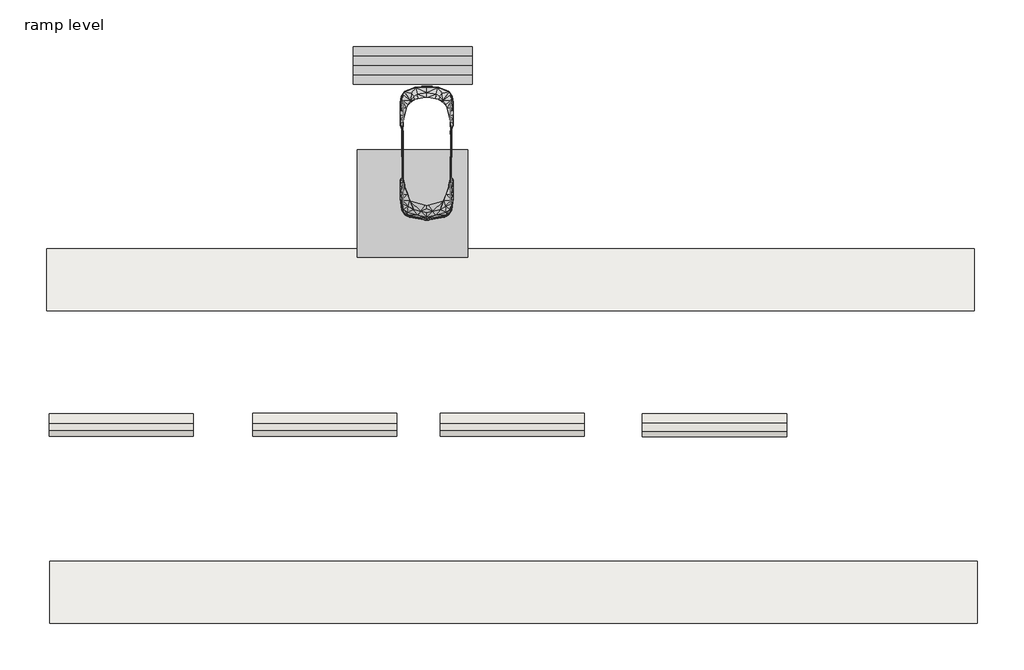
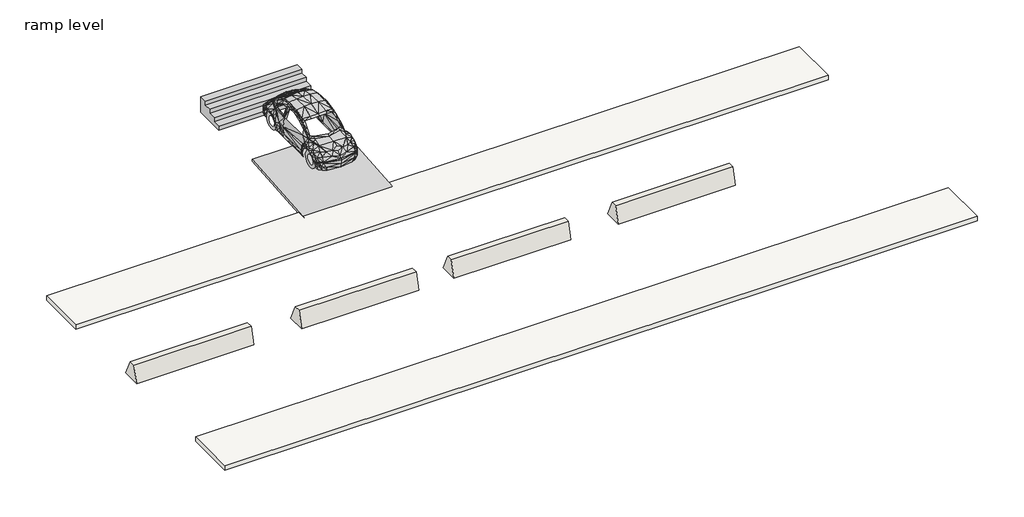
# One storey: 4 walls, 2 slabs, 1 furniture element, 1 proxy, 1 ramp.
"""IFC4 building model written with IfcOpenShell, lengths in millimetres."""

from ifc_helpers import new_model, si_unit, frame, origin, place, context, project, spatial, polyline, outline, extrude, transform, mapped, element, save
from components import rpc_beetle_rpc_beetle_31f8b51e, casework_2_casework_2_ff1f8355, ramp_2_4435543f, floors_1_floors_1_86c0a0b5, floors_2_floors_1_5c930e2b

model = new_model("IFC4")

# Units and contexts
model_context = context("Model", 3, world=origin())
ifc_project = project(units=[si_unit("LENGTHUNIT", "METRE", prefix="MILLI")], contexts=[model_context])

# Site, building, storey
site = spatial("IfcSite", under=ifc_project)
building = spatial("IfcBuilding", under=site)
storey = spatial("IfcBuildingStorey", under=building, Name="ramp level", Elevation=-304.8)

# Proxy
placement = place(None, origin())
rpc_beetle_rpc_beetle_shape = rpc_beetle_rpc_beetle_31f8b51e(model_context)
element("IfcBuildingElementProxy", 1, Name="RPC Beetle : RPC Beetle", ObjectType="RPC Beetle : RPC Beetle", at=placement, inside=storey, context=model_context, shape_type="MappedRepresentation", body=[
    mapped(rpc_beetle_rpc_beetle_shape, transform((25158.1789072, 4428.0409313, 0.0), x_axis=(-1.0, 0.0, 0.0), y_axis=(0.0, -1.0, 0.0), z_axis=(0.0, 0.0, 1.0))),
])

# Furniture
casework_2_casework_2_shape = casework_2_casework_2_ff1f8355(model_context)
element("IfcFurniture", 2, ObjectType="Casework 2 : Casework 2", at=placement, inside=storey, context=model_context, shape_type="MappedRepresentation", body=[
    mapped(casework_2_casework_2_shape, transform((0.0, -262.7690365, -6.2943409), x_axis=(1.0, 0.0, 0.0), y_axis=(0.0, 1.0, 0.0), z_axis=(0.0, 0.0, 1.0))),
])

# Ramp
ramp_2_shape = ramp_2_4435543f(model_context)
element("IfcRamp", 3, ObjectType="Ramp 2", at=placement, inside=storey, context=model_context, shape_type="MappedRepresentation", body=[
    mapped(ramp_2_shape, transform((0.0, 0.0, 0.0), x_axis=(1.0, 0.0, 0.0), y_axis=(0.0, 1.0, 0.0), z_axis=(0.0, 0.0, 1.0))),
])

# Slabs
floors_1_floors_1_shape = floors_1_floors_1_86c0a0b5(model_context)
element("IfcSlab", 4, ObjectType="Floors 1 : Floors 1", at=placement, inside=storey, context=model_context, shape_type="MappedRepresentation", body=[
    mapped(floors_1_floors_1_shape, transform((0.0, -558.8, 0.0), x_axis=(1.0, 0.0, 0.0), y_axis=(0.0, 1.0, 0.0), z_axis=(0.0, 0.0, 1.0))),
])
floors_2_floors_1_shape = floors_2_floors_1_5c930e2b(model_context)
element("IfcSlab", 5, ObjectType="Floors 2 : Floors 1", at=placement, inside=storey, context=model_context, shape_type="MappedRepresentation", body=[
    mapped(floors_2_floors_1_shape, transform((-101.6, -495.3, -133.35), x_axis=(1.0, 0.0, 0.0), y_axis=(0.0, 1.0, 0.0), z_axis=(0.0, 0.0, 1.0))),
])

# Walls
element("IfcWall", 6, at=placement, inside=storey, context=model_context, shape_type="SweptSolid", body=[
    extrude(outline(polyline([(-4504.5594538, -304.8), (-5180.7624299, -304.8), (-5017.4206022, 304.8), (-4788.8206022, 304.8), (-4504.5594538, -304.8)])), frame((13987.9647012, 0.0, 0.0), z_axis=(1.0, 0.0, 0.0), x_axis=(0.0, 1.0, 0.0)), (0.0, 0.0, 1.0), 4267.2),
])
element("IfcWall", 7, at=placement, inside=storey, context=model_context, shape_type="SweptSolid", body=[
    extrude(outline(polyline([(-4501.5479203, -304.8), (-5177.7508964, -304.8), (-5014.4090687, 304.8), (-4785.8090687, 304.8), (-4501.5479203, -304.8)])), frame((20003.9136801, 0.0, 0.0), z_axis=(1.0, 0.0, 0.0), x_axis=(0.0, 1.0, 0.0)), (0.0, 0.0, 1.0), 4267.2),
])
element("IfcWall", 8, at=placement, inside=storey, context=model_context, shape_type="SweptSolid", body=[
    extrude(outline(polyline([(-4501.5479203, -304.8), (-5177.7508964, -304.8), (-5014.4090687, 304.8), (-4785.8090687, 304.8), (-4501.5479203, -304.8)])), frame((25553.8136801, 0.0, 0.0), z_axis=(1.0, 0.0, 0.0), x_axis=(0.0, 1.0, 0.0)), (0.0, 0.0, 1.0), 4267.2),
])
element("IfcWall", 9, at=placement, inside=storey, context=model_context, shape_type="SweptSolid", body=[
    extrude(outline(polyline([(-4511.3777528, -304.8), (-5187.580729, -304.8), (-5024.2389013, 304.8), (-4795.6389013, 304.8), (-4511.3777528, -304.8)])), frame((31536.8886189, 0.0, 0.0), z_axis=(1.0, 0.0, 0.0), x_axis=(0.0, 1.0, 0.0)), (0.0, 0.0, 1.0), 4267.2),
])

save(model, "model.ifc")

# Revit data of these elements
# Type "RPC Beetle : RPC Beetle"
#   built-in parameter 1005198 = "{2, 15},{39, RPC-16-0U6E-L4EG-ENH1-J3KF-SVEL-0TX4-C0},{1, 0},{1, 0},{2, 36},{1, 8},{5, Color},{1, 0},{1, 0},{3, 0.8},{3, 0.8},{3, 0.8},{1, 8},{7, BBoxMin},{1, 0},{1, 0},{1, 0},{1, 0},{1, 0},{1, 8},{7, BBoxMax},{1, 0},{1, 0},{1, 0},{1, 0},{1, 0},{2, 11},{9, RPCTypeId},{1, 0},{1, 0},{39, RPC-16-0U6E-L4EG-ENH1-J3KF-SVEL-0TX4-C0},{1, 6},{14, RPCPlantHeight},{1, 0},{1, 0},{7, 4.91667},{2, 11},{20, AdvancedUIDefinition},{1, 0},{1, 0},{0, },{2, 11},{10, AssetLibID},{1, 0},{1, 0},{36, 4D3F6E72-3F99-4203-98E9-AF80B3C7A7A4},{2, 11},{10, BaseSchema},{1, 0},{1, 0},{9, RPCSchema},{2, 11},{12, ExchangeGUID},{1, 0},{1, 0},{0, },{1, 2},{6, Hidden},{1, 0},{1, 0},{1, 0},{2, 11},{12, LocalizedUID},{1, 0},{1, 0},{0, },{1, 4},{11, RPCCategory},{1, 0},{1, 0},{1, 0},{2, 11},{8, RPCImage},{1, 0},{1, 0},{0, },{1, 4},{13, SchemaVersion},{1, 0},{1, 0},{1, 4},{2, 11},{12, UIDefinition},{1, 0},{1, 0},{0, },{2, 11},{6, UIName},{1, 0},{1, 0},{39, RPC-16-0U6E-L4EG-ENH1-J3KF-SVEL-0TX4-C0},{2, 11},{11, VersionGUID},{1, 0},{1, 0},{9, RPCSchema},{2, 11},{9, assettype},{1, 0},{1, 0},{11, RPCGeometry},{2, 11},{11, description},{1, 0},{1, 0},{0, },{2, 11},{9, localname},{1, 0},{1, 0},{3, RPC},{2, 11},{9, localtype},{1, 0},{1, 0},{3, RPC},{1, 4},{8, revision},{1, 0},{1, 0},{1, 1},{2, 11},{9, thumbnail},{1, 0},{1, 0},{0, },{1, 4},{7, version},{1, 0},{1, 0},{1, 1},{2, 14},{6, Height},{1, 0},{1, 0},{7, 4.91667},{1, 2},{20, RPC_Cast Reflections},{1, 0},{1, 0},{1, 1},{1, 4},{16, RPC_Transparency},{1, 0},{1, 0},{2, 18},{1, 4},{11, RPC_Tinting},{1, 0},{1, 0},{2, 50},{1, 2},{15, RPC_Use Tinting},{1, 0},{1, 0},{1, 0},{1, 2},{17, RPC_License Plate},{1, 0},{1, 0},{1, 0},{2, 11},{25, RPC_License Plate Texture},{1, 0},{1, 0},{64, __RPC:/object data/textures/car/plate/textures/default/rgb/0/0/0},{2, 11},{27, RPC_i_License Plate Texture},{1, 0},{1, 0},{0, },{1, 2},{16, RPC_Custom Plate},{1, 0},{1, 0},{1, 0},{2, 11},{27, RPC_License Plate File Name},{1, 0},{1, 0},{0, },{2, 11},{7, keyword},{1, 0},{1, 0},{27, :Geometry:RPC:VW Beetle [4]},{2, 11},{8, category},{1, 0},{1, 0},{21, :Auto_Economy/Midsize},{21, assetlibrary_base.fbx},{1, 5},"
#   built-in parameter 1005195 = "RPC-16-0U6E-L4EG-ENH1-J3KF-SVEL-0TX4-C0"
#   Height = 0
# Type "Ramp 2"
#   Assembly Code = "B1010600"
#   built-in parameter 1008304 = 0.25 (stored number, unit not read)
#   built-in parameter 1008303 = 30 (stored number, unit not read)
#   built-in parameter 1008301 = 12 (stored number, unit not read)
#   Function = 0
# Type
#   Assembly Code = "B2010"
#   Layers, outside or top first: 0' - 9" no material (function 1)
# Element 1 (IfcBuildingElementProxy, "RPC Beetle : RPC Beetle")
#   Phase Created = New Construction
# Element 2 (IfcFurniture, "Casework 2 : Casework 2")
#   Phase Created = New Construction
# Element 3 (IfcRamp, "Ramp 2")
#   built-in parameter 1007275 = "DN"
#   built-in parameter 1007272 = "UP"
#   Width = 3' - 0"
#   built-in parameter 1007278 = 1
#   built-in parameter 1007276 = 1
#   built-in parameter 1007274 = 1
#   built-in parameter 1007273 = 1
#   built-in parameter 1007271 = 1
#   Phase Created = New Construction
# Element 4 (IfcSlab, "Floors 1 : Floors 1")
#   Phase Created = New Construction
#   Materials on its faces: "Concrete, Cast-in-Place gray"
# Element 5 (IfcSlab, "Floors 2 : Floors 1")
#   Phase Created = New Construction
#   Materials on its faces: "Concrete, Cast-in-Place gray"
# Elements 6, 7, 8, 9 (IfcWall)
#   Top Offset = 0' - 0"
#   Base Offset = 0' - 0"
#   Unconnected Height = 2' - 0"
#   wall height = 2' - 0"
#   Phase Created = New Construction
#   Base Constraint = ramp level
#   Materials on its faces: "Default Wall"
# Materials
#   "Concrete, Cast-in-Place gray": class "Concrete", colour RGB 192 192 192, transparency 0, Description = "Cast-in-place concrete", Cost = 0
#   "Default Wall": colour RGB 128 128 128, transparency 0, Cost = 0
